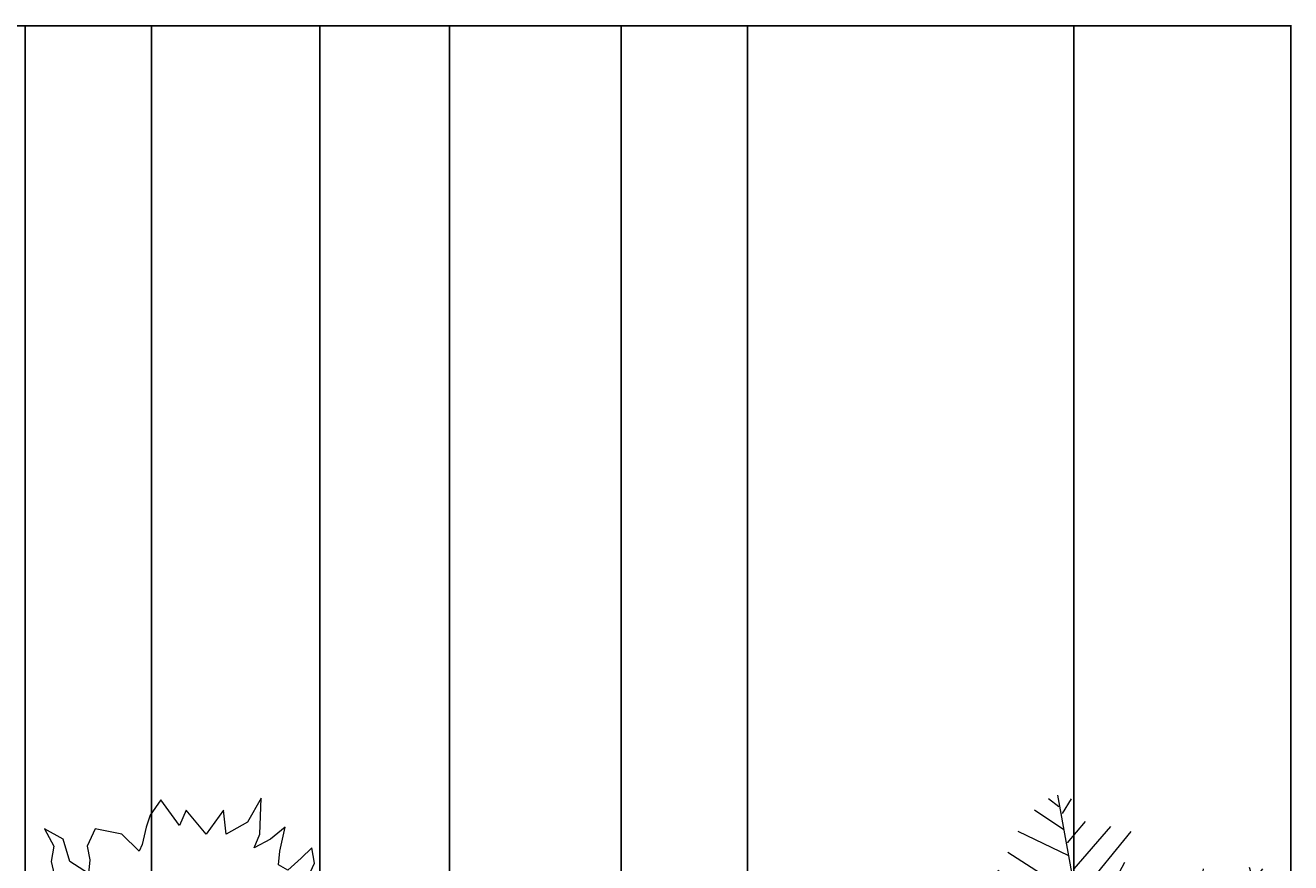
# Model space of a CAD drawing. Units: inches. Extents: x -4843 to -3402, y -164 to 3629.
# Tile 22 of 22: x -4303 to -3942, y 1154 to 1393. Entities that reach past the tile are written whole.
import ezdxf

# ---------------------------------------------------------------- set-up
doc = ezdxf.new("R2010")
doc.units = ezdxf.units.IN
doc.layers.add('A-ANNO-DIMS', color=2, linetype='Continuous', lineweight=18)
doc.layers.add('PLANTS', color=3, linetype='Continuous', lineweight=13)
doc.styles.get("Standard").update_dxf_attribs({"font": 'arial.ttf'})
doc.dimstyles.get("Standard").update_dxf_attribs({"dimtxt": 0.18, "dimasz": 0.18, "dimexe": 0.18, "dimexo": 0.0625, "dimgap": 0.09, "dimtad": 0, "dimtih": 1, "dimtoh": 1, "dimdec": 4, "dimzin": 0, "dimdsep": 46, "dimtxsty": 'Standard', "dimcen": 0.09, "dimadec": 0, "dimazin": 0, "dimtfac": 1, "dimtdec": 4, "dimtofl": 0, "dimtmove": 0, "dimatfit": 3, "dimfxl": 1, "dimtolj": 1, "dimtzin": 0, "dimarcsym": 0})

# ---------------------------------------------------------------- blocks, each defined once
blk = doc.blocks.new('*U33')
for p, q in [((-258.7244, 1362.456), (-332.3336, 1421.4348)), ((0, 0), (-266.7, 1447.8)), ((-231.1146, 1315.2628), (-166.7002, 1421.4348)), ((-221.9198, 1197.3052), (-433.5526, 1338.8594)), ((-194.31, 1102.9442), (-65.4812, 1256.284)), ((-148.3106, 914.1968), (118.5418, 1220.9018)), ((-185.1152, 1008.5578), (-553.1612, 1185.4942)), ((-129.8956, 701.8528), (265.7602, 1185.4942)), ((-129.8956, 713.6638), (-626.7704, 1032.1544)), ((-74.7014, 418.7444), (219.7608, 961.39)), ((1121.4862, 925.9824), (1149.0706, 831.6214)), ((-93.091, 489.5342), (-700.3796, 902.3858)), ((685.8, 228.6), (1219.2, 914.4)), ((689.0258, 230.0224), (790.2448, 914.1968)), ((891.4384, 831.6214), (946.658, 572.1096)), ((983.4626, 867.0036), (1066.2666, 725.4494)), ((-1234.059, 536.7274), (-1252.4486, 737.2604)), ((412.9786, 147.447), (587.8068, 796.2392)), ((560.197, 182.8292), (698.2206, 819.8358)), ((808.6344, 784.4282), (827.0494, 418.7444)), ((1112.2914, 760.8316), (1296.3144, 784.4282)), ((-800.1, 114.3), (-1333.5, 647.7)), ((-1105.2302, 725.4494), (-1077.6458, 395.1732)), ((-976.4268, 666.4706), (-884.4026, 194.6402)), ((-902.8176, 713.6638), (-617.5756, 100.2538)), ((-369.1382, 53.086), (-783.1836, 642.874)), ((-28.6766, 171.0436), (228.9556, 678.2816)), ((256.5654, 88.4682), (449.7832, 666.4706)), ((1029.462, 654.685), (1241.0948, 631.0884)), ((-617.5756, 607.4918), (-74.7014, 347.98)), ((100.1268, 41.275), (284.1498, 619.2774)), ((-1206.4492, 501.3198), (-1418.082, 465.9376)), ((919.0482, 501.3198), (1222.6798, 454.152)), ((845.439, 418.7444), (1241.0948, 277.1902)), ((-1031.621, 347.98), (-1399.667, 277.1902)), ((-525.5514, 347.98), (-28.6766, 123.8504)), ((753.4148, 312.5978), (1222.6798, 159.2326)), ((0, 0), (685.8, 228.6)), ((615.4166, 194.6402), (1185.8752, 41.275)), ((-847.598, 159.2326), (-1326.0578, 135.636)), ((0, 0), (-800.1, 114.3)), ((458.978, 147.447), (891.4384, -88.4682)), ((-718.7946, 88.4682), (-1215.644, -147.447)), ((-543.9664, 76.6572), (-967.2066, -206.4512)), ((-405.9428, 53.086), (-764.794, -241.8334)), ((0, 0), (-571.5, -495.3)), ((-166.7002, 29.4894), (-543.9664, -206.4512)), ((0, 0), (457.2, -571.5)), ((164.5412, 41.275), (661.416, -218.2368)), ((284.1498, 88.4682), (781.0246, -147.447)), ((-120.7008, -88.4682), (-93.091, -371.5766)), ((63.3222, -76.6826), (-37.8714, -513.1308)), ((44.9326, -64.897), (615.4166, -241.8334)), ((-166.7002, -147.447), (-507.1618, -253.619)), ((127.7366, -159.258), (54.1274, -654.685)), ((-240.3094, -218.2368), (-157.5054, -595.7062)), ((192.151, -230.0224), (817.8292, -371.5766)), ((-387.5278, -324.4088), (-764.794, -324.4088)), ((-341.5284, -289.0012), (-221.9198, -831.6214)), ((228.9556, -289.0012), (90.932, -914.1968)), ((-442.7474, -383.3876), (-1086.8406, -477.7486)), ((-433.5526, -383.3876), (-323.1134, -1020.3688)), ((357.759, -430.5554), (164.5412, -1020.3688)), ((311.7596, -383.3876), (937.4378, -477.7486)), ((-617.5756, -548.5384), (-1077.6458, -560.324)), ((-571.5, -495.3), (-952.5, -1143)), ((-525.5514, -465.963), (-451.9422, -1126.5408)), ((412.9786, -501.3452), (919.0482, -583.9206)), ((-635.9652, -607.5172), (-580.771, -1150.1374)), ((458.978, -572.1096), (210.5406, -1161.923)), ((457.2, -571.5), (685.8, -1333.5)), ((468.1982, -572.1096), (1029.462, -737.2604)), ((-681.9646, -666.496), (-1022.4262, -654.685)), ((486.5878, -642.8994), (983.4626, -843.4324)), ((-718.7946, -737.2604), (-1086.8406, -796.2392)), ((-737.1842, -784.4536), (-709.5744, -1114.7298)), ((514.1976, -772.6426), (403.7838, -1138.3264)), ((-783.1836, -867.029), (-1077.6458, -902.4112)), ((541.8074, -831.6214), (992.6574, -1032.1544)), ((-875.2078, -1008.5832), (-1040.8412, -1079.3476)), ((-829.2084, -937.7934), (-810.7934, -1126.5408)), ((578.612, -961.39), (495.7826, -1232.7128)), ((578.612, -973.1756), (873.0488, -1138.3264)), ((624.6114, -1161.923), (587.8068, -1291.6916)), ((624.6114, -1102.9442), (781.0246, -1209.1162)), ((679.8056, -1268.095), (716.6102, -1291.6916))]:
    blk.add_line(p, q)
blk = doc.blocks.new('*U34')
for points in [[(0, 1540.256), (-77.4954, 1428.4452), (-106.5784, 1341.501), (-135.636, 1217.295), (-155.0162, 1167.6126), (-280.9748, 1291.8186), (-474.7514, 1329.0804), (-532.892, 1204.8744), (-513.5118, 1105.5096), (-523.1892, 1006.1194), (-658.8506, 1093.089), (-707.2884, 1254.5568), (-842.9244, 1329.0804), (-775.1064, 1204.8744), (-794.4866, 1093.089), (-765.429, 968.8576), (-852.6272, 894.334), (-1036.701, 931.5958), (-1249.8832, 968.8576), (-1191.7426, 931.5958), (-1075.4614, 807.3898), (-1075.4614, 720.4456), (-1182.0398, 695.6044), (-1414.5768, 695.6044), (-1269.238, 558.9524), (-1385.5192, 534.1112), (-1172.3624, 372.6434), (-1307.9984, 285.6992), (-1521.1552, 285.6992), (-1414.5768, 223.5962), (-1366.139, 136.652), (-1453.3372, 86.9442), (-1540.5354, -37.2618), (-1550.2382, -124.206), (-1501.775, -86.9442), (-1385.5192, -37.2618), (-1307.9984, -111.7854), (-1346.7588, -260.8326), (-1501.775, -385.064), (-1249.8832, -335.3816), (-1482.3948, -621.0554), (-1230.503, -534.1112), (-1104.5444, -571.373), (-1094.8416, -658.3172), (-1201.42, -794.9692), (-1094.8416, -770.128), (-1230.503, -1006.1194), (-978.5858, -807.3898), (-1036.701, -919.1752), (-823.5442, -944.0164), (-852.6272, -1105.4842), (-901.065, -1254.5568), (-726.6686, -1142.746), (-600.71, -1180.0078), (-561.9496, -1316.6598), (-552.2722, -1465.707), (-484.4542, -1329.0804), (-397.2306, -1316.6598), (-319.7352, -1490.5482), (-280.9748, -1391.1834), (-174.3964, -1254.5568), (-174.3964, -1353.9216), (-125.9586, -1229.7156), (-48.4378, -1565.0718), (-29.0576, -1304.2392), (116.2812, -1502.9688), (135.6614, -1378.7628), (251.9172, -1440.8658), (310.0578, -1540.2306), (329.438, -1217.295), (377.8758, -1130.3254), (445.6938, -1204.8744), (494.157, -1341.501), (581.3552, -1540.2306), (552.2722, -1254.5568), (600.71, -1180.0078), (755.7516, -1217.295), (891.3876, -1329.0804), (939.8254, -1366.3422), (842.9498, -1180.0078), (813.8668, -1055.8018), (891.3876, -993.6988), (1114.2472, -1030.9606), (1211.1228, -1068.2224), (1094.867, -919.1752), (1094.867, -857.0722), (1182.0652, -794.9692), (1278.9408, -832.231), (1191.7426, -670.7378), (1414.6022, -571.373), (1540.5608, -583.7936), (1685.8996, -558.9524), (1521.1806, -509.27), (1375.8418, -459.5876), (1317.7012, -397.4846), (1259.5606, -310.515), (1308.0238, -260.8326), (1472.7174, -248.412), (1608.3788, -186.309), (1637.4364, -74.5236)], [(1647.1392, -74.5236), (1511.4778, -136.6266), (1433.9824, -111.7854), (1317.7012, -62.103), (1327.404, 24.8412), (1404.8994, 99.3648), (1521.1806, 149.0726), (1598.676, 285.6992), (1482.4202, 260.858), (1385.5192, 260.858), (1298.321, 285.6992), (1366.139, 397.4846), (1472.7174, 459.5876), (1540.5608, 496.8494), (1424.2796, 496.8494), (1298.321, 447.167), (1182.0652, 484.4288), (1172.3624, 571.3984), (1259.5606, 695.6044), (1327.404, 881.9134), (1259.5606, 857.0722), (1123.9246, 770.128), (1046.4038, 819.8104), (1056.1066, 956.437), (1114.2472, 1080.6684), (1094.867, 1192.4538), (1017.3462, 1117.9302), (920.4452, 1030.9606), (852.6272, 1068.2478), (862.33, 1167.6126), (901.0904, 1341.501), (794.512, 1254.5568), (678.2308, 1192.4538), (716.9912, 1291.8186), (726.6686, 1552.6766), (629.793, 1378.7628), (474.7768, 1291.8186), (455.3966, 1465.7324), (329.438, 1291.8186), (184.0992, 1465.7324), (135.6614, 1353.9216), (0, 1540.256)]]:
    blk.add_lwpolyline(points)
blk.add_lwpolyline([(9.7028, 49.6824), (0, 0), (48.4378, 12.4206), (58.1406, 37.2618)], close=True)
blk = doc.blocks.new('*D60')
at = {"layer": 'A-ANNO-DIMS', "color": 0, "lineweight": -2, "transparency": 16777216}
for p, q in [((-4723.78, 1149.42), (-4723.78, 1392.95)), ((-4723.6, 1392.77), (-4333.07, 1392.77)), ((-3941.96, 1392.77), (-4332.5, 1392.77)), ((-3941.78, 1149.42), (-3941.78, 1392.95))]:
    blk.add_line(p, q, dxfattribs=at)
at = {"layer": 'A-ANNO-DIMS', "color": 0, "transparency": 16777216}
for points in [[(-4723.6, 1392.8), (-4723.6, 1392.74), (-4723.78, 1392.77)], [(-3941.96, 1392.8), (-3941.96, 1392.74), (-3941.78, 1392.77)]]:
    blk.add_solid(points, dxfattribs=at)
at = {"layer": 'Defpoints', "color": 0, "transparency": 16777216}
for p in [(-3941.78, 1392.77), (-4723.78, 1149.35), (-3941.78, 1149.35)]:
    blk.add_point(p, dxfattribs=at)
at = {"layer": 'A-ANNO-DIMS', "color": 0, "transparency": 16777216, "insert": (-4332.78, 1392.77), "char_height": 0.18, "attachment_point": 5}
blk.add_mtext('\\A1;782', dxfattribs=at)
blk = doc.blocks.new('*D72')
at = {"layer": 'A-ANNO-DIMS', "color": 0, "lineweight": -2, "transparency": 16777216}
for p, q in [((-4302.78, 1011.42), (-4302.78, 1392.95)), ((-4302.6, 1392.77), (-4285, 1392.77)), ((-4266.96, 1392.77), (-4284.56, 1392.77)), ((-4266.78, 1020.42), (-4266.78, 1392.95))]:
    blk.add_line(p, q, dxfattribs=at)
at = {"layer": 'A-ANNO-DIMS', "color": 0, "transparency": 16777216}
for points in [[(-4302.6, 1392.8), (-4302.6, 1392.74), (-4302.78, 1392.77)], [(-4266.96, 1392.8), (-4266.96, 1392.74), (-4266.78, 1392.77)]]:
    blk.add_solid(points, dxfattribs=at)
at = {"layer": 'Defpoints', "color": 0, "transparency": 16777216}
for p in [(-4266.78, 1392.77), (-4266.78, 1020.35), (-4302.78, 1011.35)]:
    blk.add_point(p, dxfattribs=at)
at = {"layer": 'A-ANNO-DIMS', "color": 0, "transparency": 16777216, "insert": (-4284.78, 1392.77), "char_height": 0.18, "attachment_point": 5}
blk.add_mtext('\\A1;36', dxfattribs=at)
blk = doc.blocks.new('*D79')
at = {"layer": 'A-ANNO-DIMS', "color": 0, "lineweight": -2, "transparency": 16777216}
for p, q in [((-4132.78, 965.42), (-4132.78, 1392.95)), ((-4132.6, 1392.77), (-4115, 1392.77)), ((-4096.96, 1392.77), (-4114.56, 1392.77)), ((-4096.78, 965.42), (-4096.78, 1392.95))]:
    blk.add_line(p, q, dxfattribs=at)
at = {"layer": 'A-ANNO-DIMS', "color": 0, "transparency": 16777216}
for points in [[(-4132.6, 1392.8), (-4132.6, 1392.74), (-4132.78, 1392.77)], [(-4096.96, 1392.8), (-4096.96, 1392.74), (-4096.78, 1392.77)]]:
    blk.add_solid(points, dxfattribs=at)
at = {"layer": 'Defpoints', "color": 0, "transparency": 16777216}
for p in [(-4096.78, 1392.77), (-4132.78, 965.35), (-4096.78, 965.35)]:
    blk.add_point(p, dxfattribs=at)
at = {"layer": 'A-ANNO-DIMS', "color": 0, "transparency": 16777216, "insert": (-4114.78, 1392.77), "char_height": 0.18, "attachment_point": 5}
blk.add_mtext('\\A1;36', dxfattribs=at)
blk = doc.blocks.new('*D80')
at = {"layer": 'A-ANNO-DIMS', "color": 0, "lineweight": -2, "transparency": 16777216}
for p, q in [((-4218.78, 1020.42), (-4218.78, 1392.95)), ((-4218.6, 1392.77), (-4200.5, 1392.77)), ((-4181.96, 1392.77), (-4200.06, 1392.77)), ((-4181.78, 1020.42), (-4181.78, 1392.95))]:
    blk.add_line(p, q, dxfattribs=at)
at = {"layer": 'A-ANNO-DIMS', "color": 0, "transparency": 16777216}
for points in [[(-4218.6, 1392.8), (-4218.6, 1392.74), (-4218.78, 1392.77)], [(-4181.96, 1392.8), (-4181.96, 1392.74), (-4181.78, 1392.77)]]:
    blk.add_solid(points, dxfattribs=at)
at = {"layer": 'Defpoints', "color": 0, "transparency": 16777216}
for p in [(-4181.78, 1392.77), (-4218.78, 1020.35), (-4181.78, 1020.35)]:
    blk.add_point(p, dxfattribs=at)
at = {"layer": 'A-ANNO-DIMS', "color": 0, "transparency": 16777216, "insert": (-4200.28, 1392.77), "char_height": 0.18, "attachment_point": 5}
blk.add_mtext('\\A1;37', dxfattribs=at)
blk = doc.blocks.new('*D81')
at = {"layer": 'A-ANNO-DIMS', "color": 0, "lineweight": -2, "transparency": 16777216}
for p, q in [((-4332.78, 86.42), (-4332.78, 1392.95)), ((-4332.6, 1392.77), (-4168.61, 1392.77)), ((-4003.86, 1392.77), (-4167.86, 1392.77)), ((-4003.68, 86.42), (-4003.68, 1392.95))]:
    blk.add_line(p, q, dxfattribs=at)
at = {"layer": 'A-ANNO-DIMS', "color": 0, "transparency": 16777216}
for points in [[(-4332.6, 1392.8), (-4332.6, 1392.74), (-4332.78, 1392.77)], [(-4003.86, 1392.8), (-4003.86, 1392.74), (-4003.68, 1392.77)]]:
    blk.add_solid(points, dxfattribs=at)
at = {"layer": 'Defpoints', "color": 0, "transparency": 16777216}
for p in [(-4003.68, 1392.77), (-4332.78, 86.35), (-4003.68, 86.35)]:
    blk.add_point(p, dxfattribs=at)
at = {"layer": 'A-ANNO-DIMS', "color": 0, "transparency": 16777216, "insert": (-4168.23, 1392.77), "char_height": 0.18, "attachment_point": 5}
blk.add_mtext('\\A1;329.1', dxfattribs=at)

msp = doc.modelspace()

# ---------------------------------------------------------------- block references
at = {"layer": 'PLANTS', "xscale": 0.0393700787401575, "yscale": 0.0393700787401575, "zscale": 0.0393700787401575}
for name, p in [('*U33', (-3997.76, 1116.35)), ('*U34', (-4264.15, 1111.38))]:
    msp.add_blockref(name, p, dxfattribs=at)

# ---------------------------------------------------------------- dimensions: what is measured, and where the dimension line sits
at = {"layer": 'A-ANNO-DIMS'}
for base, p1, p2, override, picture, middle in [((-3941.78, 1392.77), (-4723.78, 1149.35), (-3941.78, 1149.35), {"dimdec": 0, "dimlfac": 1, "dimrnd": 0, "dimzin": 0, "dimdsep": 46, "dimlunit": 2}, '*D60', (-4332.78, 1392.77)), ((-4003.68, 1392.77), (-4332.78, 86.35), (-4003.68, 86.35), {"dimdec": 1, "dimlfac": 1, "dimrnd": 0, "dimzin": 0, "dimdsep": 46, "dimlunit": 2}, '*D81', (-4168.23, 1392.77)), ((-4266.78, 1392.77), (-4302.78, 1011.35), (-4266.78, 1020.35), {"dimdec": 0, "dimlfac": 1, "dimrnd": 0, "dimzin": 0, "dimdsep": 46, "dimlunit": 2}, '*D72', (-4284.78, 1392.77)), ((-4181.78, 1392.77), (-4218.78, 1020.35), (-4181.78, 1020.35), {"dimdec": 0, "dimlfac": 1, "dimrnd": 0, "dimzin": 0, "dimdsep": 46, "dimlunit": 2}, '*D80', (-4200.28, 1392.77)), ((-4096.78, 1392.77), (-4132.78, 965.35), (-4096.78, 965.35), {"dimdec": 0, "dimlfac": 1, "dimrnd": 0, "dimzin": 0, "dimdsep": 46, "dimlunit": 2}, '*D79', (-4114.78, 1392.77))]:
    dim = msp.add_linear_dim(base=base, p1=p1, p2=p2, dimstyle='Standard', override=override, dxfattribs=at)
    dim.commit()
    dim.dimension.update_dxf_attribs({"geometry": picture, "text_midpoint": middle})

doc.saveas('drawing.dxf')
